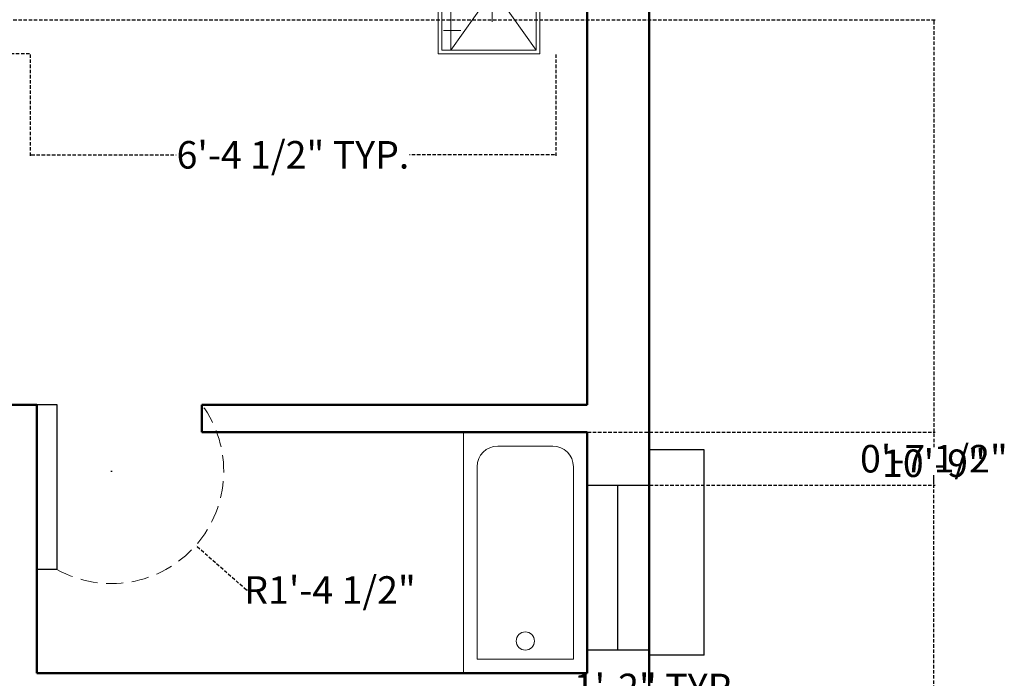
# Model space of a CAD drawing. Units: inches. Extents: x 513 to 1142, y 396 to 927.
# Tile 28 of 31: x 998 to 1142, y 674 to 770. Entities that reach past the tile are written whole.
import ezdxf

# ---------------------------------------------------------------- set-up
doc = ezdxf.new("R2010")
doc.units = ezdxf.units.IN
doc.header["$MEASUREMENT"] = 0
doc.linetypes.add('DASHED', pattern=[0.75, 0.5, -0.25])
for name, color, linetype, lineweight in [('A-ANNO-DIMS', 2, 'DASHED', 18), ('A-DOOR', 4, 'Continuous', 25), ('A-DOOR-SWNG', 4, 'DASHED', 13), ('A-FLOR-FIXT', 92, 'Continuous', 18), ('A-WALL', 7, 'Continuous', 50), ('furniture', 92, 'Continuous', 18), ('windows', 172, 'Continuous', 25)]:
    doc.layers.add(name, color=color, linetype=linetype, lineweight=lineweight)
doc.styles.get("Standard").update_dxf_attribs({"font": 'arial.ttf'})
doc.dimstyles.get("Standard").update_dxf_attribs({"dimtxt": 4, "dimasz": 0.18, "dimexe": 0.18, "dimexo": 0.0625, "dimgap": 0.09, "dimtad": 0, "dimtih": 1, "dimtoh": 1, "dimdec": 0, "dimrnd": 6, "dimzin": 0, "dimdsep": 46, "dimlunit": 3, "dimtxsty": 'Standard', "dimcen": 0.09, "dimadec": 0, "dimazin": 0, "dimtfac": 1, "dimtdec": 0, "dimtofl": 0, "dimtmove": 0, "dimatfit": 3, "dimfxl": 1, "dimtolj": 1, "dimtzin": 0, "dimarcsym": 0})

# ---------------------------------------------------------------- blocks, each defined once
blk = doc.blocks.new('A$C029D5C69')
for p, q in [((2.6479, 2.0066), (2.1429, 2.0066)), ((2.6328, 1.9915), (2.158, 1.9915)), ((2.6328, 1.6211), (2.6328, 1.9915)), ((2.6479, 1.606), (2.6479, 2.0066)), ((2.2367, 1.8186), (2.5212, 1.8186)), ((2.5551, 1.6275), (2.5551, 1.696)), ((2.1429, 1.606), (2.6479, 1.606)), ((2.158, 1.6211), (2.6328, 1.6211))]:
    blk.add_line(p, q)
at = {"ltscale": 0.005}
for p, q in [((2.6328, 1.6568), (2.158, 1.9915)), ((2.158, 1.6568), (2.6328, 1.9915)), ((2.6328, 1.6568), (2.158, 1.6568))]:
    blk.add_line(p, q, dxfattribs=at)
blk = doc.blocks.new('A$C0D3A6DFA')
blk.add_blockref('A$C029D5C69', (0, 0))
blk = doc.blocks.new('WIN-24IN')
blk.add_line((0, 4.39), (24, 4.39))
blk.add_lwpolyline([(24, 0), (0, 0), (0, 9), (24, 9)], close=True)
blk = doc.blocks.new('DOOR-LEAF-24IN')
blk.add_lwpolyline([(3, 24), (3, 0), (0, 0), (0, 24)], close=True)
blk = doc.blocks.new('BASIN-BOWL-14X31')
for p, q in [((11, 31), (3, 31)), ((0, 0), (0, 28)), ((14, 0), (14, 28)), ((0, 0), (14, 0))]:
    blk.add_line(p, q)
for centre, start, end in [((3, 28), 90, 180), ((11, 28), 0, 90)]:
    blk.add_arc(centre, 3, start, end)
blk = doc.blocks.new('*D117')
at = {"layer": 'A-ANNO-DIMS', "color": 0, "lineweight": -2, "transparency": 16777216}
for p, q in [((999.94, 862.98), (985.15, 862.98)), ((985.33, 862.8), (985.33, 816.24)), ((985.33, 765.36), (985.33, 811.92)), ((999.94, 765.18), (985.15, 765.18))]:
    blk.add_line(p, q, dxfattribs=at)
at = {"layer": 'A-ANNO-DIMS', "color": 0, "transparency": 16777216}
for points in [[(985.3, 862.8), (985.36, 862.8), (985.33, 862.98)], [(985.3, 765.36), (985.36, 765.36), (985.33, 765.18)]]:
    blk.add_solid(points, dxfattribs=at)
at = {"layer": 'Defpoints', "color": 0, "transparency": 16777216}
for p in [(1000, 862.98), (985.33, 765.18), (1000, 765.18)]:
    blk.add_point(p, dxfattribs=at)
at = {"layer": 'A-ANNO-DIMS', "color": 0, "transparency": 16777216, "insert": (985.33, 814.08), "char_height": 4, "attachment_point": 5}
blk.add_mtext('\\A1;BED GROUP 8\'-2" TYP.', dxfattribs=at)
blk = doc.blocks.new('*D118')
at = {"layer": 'A-ANNO-DIMS', "color": 0, "lineweight": -2, "transparency": 16777216}
for p, q in [((1000, 765.12), (1000, 750.33)), ((1076.43, 765.12), (1076.43, 750.33)), ((1000.18, 750.51), (1021.26, 750.51)), ((1076.25, 750.51), (1055.17, 750.51))]:
    blk.add_line(p, q, dxfattribs=at)
at = {"layer": 'A-ANNO-DIMS', "color": 0, "transparency": 16777216}
for points in [[(1000.18, 750.54), (1000.18, 750.48), (1000, 750.51)], [(1076.25, 750.54), (1076.25, 750.48), (1076.43, 750.51)]]:
    blk.add_solid(points, dxfattribs=at)
at = {"layer": 'Defpoints', "color": 0, "transparency": 16777216}
for p in [(1000, 765.18), (1076.43, 765.18), (1076.43, 750.51)]:
    blk.add_point(p, dxfattribs=at)
at = {"layer": 'A-ANNO-DIMS', "color": 0, "transparency": 16777216, "insert": (1038.22, 750.51), "char_height": 4, "attachment_point": 5}
blk.add_mtext('\\A1;6\'-4 1/2" TYP.', dxfattribs=at)
blk = doc.blocks.new('*D132')
at = {"layer": 'A-ANNO-DIMS', "color": 0, "lineweight": -2, "transparency": 16777216}
for p, q in [((1065, 669.22), (1065, 673.24)), ((1065.18, 673.06), (1078.82, 673.06)), ((1079, 669.22), (1079, 673.24)), ((1079, 673.06), (1079.18, 673.06))]:
    blk.add_line(p, q, dxfattribs=at)
at = {"layer": 'A-ANNO-DIMS', "color": 0, "transparency": 16777216}
for points in [[(1065.18, 673.09), (1065.18, 673.03), (1065, 673.06)], [(1078.82, 673.09), (1078.82, 673.03), (1079, 673.06)]]:
    blk.add_solid(points, dxfattribs=at)
at = {"layer": 'Defpoints', "color": 0, "transparency": 16777216}
for p in [(1079, 673.06), (1065, 669.16), (1079, 669.16)]:
    blk.add_point(p, dxfattribs=at)
at = {"layer": 'A-ANNO-DIMS', "color": 0, "transparency": 16777216, "insert": (1091.27, 673.06), "char_height": 4, "attachment_point": 5}
blk.add_mtext('\\A1;1\'-2" TYP.', dxfattribs=at)
blk = doc.blocks.new('*D149')
at = {"layer": 'A-ANNO-DIMS', "color": 0, "lineweight": -2, "transparency": 16777216}
for p, q in [((840.06, 770.16), (1131.58, 770.16)), ((1131.4, 769.98), (1131.4, 707.79)), ((1131.4, 641.34), (1131.4, 703.53)), ((840.06, 641.16), (1131.58, 641.16))]:
    blk.add_line(p, q, dxfattribs=at)
at = {"layer": 'A-ANNO-DIMS', "color": 0, "transparency": 16777216}
for points in [[(1131.37, 769.98), (1131.43, 769.98), (1131.4, 770.16)], [(1131.37, 641.34), (1131.43, 641.34), (1131.4, 641.16)]]:
    blk.add_solid(points, dxfattribs=at)
at = {"layer": 'Defpoints', "color": 0, "transparency": 16777216}
for p in [(840, 770.16), (1131.4, 770.16), (840, 641.16)]:
    blk.add_point(p, dxfattribs=at)
at = {"layer": 'A-ANNO-DIMS', "color": 0, "transparency": 16777216, "insert": (1131.4, 705.66), "char_height": 4, "attachment_point": 5}
blk.add_mtext('\\A1;10\'-9"', dxfattribs=at)
blk = doc.blocks.new('*D165')
at = {"layer": 'A-ANNO-DIMS', "color": 0, "lineweight": -2, "transparency": 16777216}
for p, q in [((1081.06, 710.16), (1131.58, 710.16)), ((1131.4, 709.98), (1131.4, 708.48)), ((1131.4, 702.66), (1131.4, 704.16)), ((1081.07, 702.48), (1131.58, 702.48))]:
    blk.add_line(p, q, dxfattribs=at)
at = {"layer": 'A-ANNO-DIMS', "color": 0, "transparency": 16777216}
for points in [[(1131.37, 709.98), (1131.43, 709.98), (1131.4, 710.16)], [(1131.37, 702.66), (1131.43, 702.66), (1131.4, 702.48)]]:
    blk.add_solid(points, dxfattribs=at)
at = {"layer": 'Defpoints', "color": 0, "transparency": 16777216}
for p in [(1081, 710.16), (1081, 702.48), (1131.4, 702.48)]:
    blk.add_point(p, dxfattribs=at)
at = {"layer": 'A-ANNO-DIMS', "color": 0, "transparency": 16777216, "insert": (1131.4, 706.32), "char_height": 4, "attachment_point": 5}
blk.add_mtext('\\A1;0\'-7 1/2"', dxfattribs=at)
blk = doc.blocks.new('*D190')
at = {"layer": 'A-ANNO-DIMS', "color": 0, "lineweight": -2, "transparency": 16777216}
for p, q in [((1011.74, 704.49), (1011.92, 704.49)), ((1011.83, 704.4), (1011.83, 704.58)), ((1031.45, 687.23), (1024.23, 693.58)), ((1031.63, 687.23), (1031.45, 687.23))]:
    blk.add_line(p, q, dxfattribs=at)
at = {"layer": 'A-ANNO-DIMS', "color": 0, "transparency": 16777216}
blk.add_solid([(1024.25, 693.61), (1024.21, 693.56), (1024.09, 693.7)], dxfattribs=at)
at = {"layer": 'Defpoints', "color": 0, "transparency": 16777216}
for p in [(1011.83, 704.49), (1024.09, 693.7)]:
    blk.add_point(p, dxfattribs=at)
at = {"layer": 'A-ANNO-DIMS', "color": 0, "transparency": 16777216, "insert": (1043.61, 687.23), "char_height": 4, "attachment_point": 5}
blk.add_mtext('\\A1;R1\'-4 1/2"', dxfattribs=at)

msp = doc.modelspace()

# ---------------------------------------------------------------- linework, layer by layer
at = {"layer": 'A-DOOR-SWNG', "ltscale": 5}
msp.add_arc((1011.83, 704.49), 16.33, 240.9987, 36.2929, dxfattribs=at)
at = {"layer": 'A-FLOR-FIXT'}
msp.add_line((1063, 675.16), (1063, 710.16), dxfattribs=at)
msp.add_lwpolyline([(1081, 710.16), (1081, 710.16), (1081, 675.16), (1081, 675.16)], close=True, dxfattribs=at)
msp.add_circle((1072, 679.81), 1.33, dxfattribs=at)
at = {"layer": 'A-WALL'}
for p, q in [((1090, 431.16), (1090, 879.16)), ((1081, 714.16), (1081, 870.16)), ((1001, 714.16), (961, 714.16)), ((1001, 675.16), (1001, 714.16)), ((1081, 714.16), (1025, 714.16)), ((1025, 710.16), (1025, 714.16)), ((1081, 710.16), (1025, 710.16)), ((1081, 675.16), (1081, 710.16)), ((1001, 675.16), (1081, 675.16))]:
    msp.add_line(p, q, dxfattribs=at)
at = {"layer": 'windows'}
for p, q in [((1098, 707.63), (1090, 707.63)), ((1098, 677.77), (1098, 707.63)), ((1098, 677.77), (1090, 677.77))]:
    msp.add_line(p, q, dxfattribs=at)

# ---------------------------------------------------------------- block references
at = {"layer": 'A-DOOR'}
msp.add_blockref('DOOR-LEAF-24IN', (1000.92, 690.21), dxfattribs=at)
at = {"layer": 'A-FLOR-FIXT'}
msp.add_blockref('BASIN-BOWL-14X31', (1064.99, 677.16), dxfattribs=at)
at = {"layer": 'furniture', "xscale": 36.93602985360944, "yscale": 36.93602985360944, "zscale": 36.93602985360944, "rotation": 270}
msp.add_blockref('A$C0D3A6DFA', (1000, 862.98), dxfattribs=at)
at = {"layer": 'windows', "rotation": 269.9999999999989}
msp.add_blockref('WIN-24IN', (1081, 702.48), dxfattribs=at)

# ---------------------------------------------------------------- dimensions: what is measured, and where the dimension line sits
at = {"layer": 'A-ANNO-DIMS'}
dim = msp.add_linear_dim(base=(985.33, 765.18), p1=(1000, 862.98), p2=(1000, 765.18), angle=270, text='BED GROUP <> TYP.', dimstyle='Standard', override={"dimdec": 1, "dimlfac": 1, "dimrnd": 0, "dimzin": 1, "dimdsep": 46, "dimlunit": 4, "dimfrac": 2}, dxfattribs=at)
dim.commit()
dim.dimension.update_dxf_attribs({"geometry": '*D117', "text_midpoint": (985.33, 814.08)})
for base, p1, p2, picture, middle in [((1131.4, 770.16), (840, 641.16), (840, 770.16), '*D149', (1131.4, 705.66)), ((1131.4, 702.48), (1081, 710.16), (1081, 702.48), '*D165', (1131.4, 706.32))]:
    dim = msp.add_linear_dim(base=base, p1=p1, p2=p2, angle=90, dimstyle='Standard', override={"dimdec": 1, "dimlfac": 1, "dimrnd": 0, "dimzin": 1, "dimdsep": 46, "dimlunit": 4, "dimfrac": 2}, dxfattribs=at)
    dim.commit()
    dim.dimension.update_dxf_attribs({"geometry": picture, "text_midpoint": middle})
for base, p1, p2, picture, middle in [((1076.43, 750.51), (1000, 765.18), (1076.43, 765.18), '*D118', (1038.22, 750.51)), ((1079, 673.06), (1065, 669.16), (1079, 669.16), '*D132', (1091.27, 673.06))]:
    dim = msp.add_linear_dim(base=base, p1=p1, p2=p2, text='<> TYP.', dimstyle='Standard', override={"dimdec": 1, "dimlfac": 1, "dimrnd": 0, "dimzin": 1, "dimdsep": 46, "dimlunit": 4, "dimfrac": 2}, dxfattribs=at)
    dim.commit()
    dim.dimension.update_dxf_attribs({"geometry": picture, "text_midpoint": middle})
dim = msp.add_radius_dim(center=(1011.83, 704.49), mpoint=(1024.09, 693.7), dimstyle='Standard', override={"dimdec": 1, "dimlfac": 1, "dimrnd": 0, "dimzin": 1, "dimdsep": 46, "dimlunit": 4, "dimfrac": 2}, dxfattribs=at)
dim.commit()
dim.dimension.update_dxf_attribs({"geometry": '*D190', "text_midpoint": (1043.61, 687.23), "dimtype": 164})

doc.saveas('drawing.dxf')
